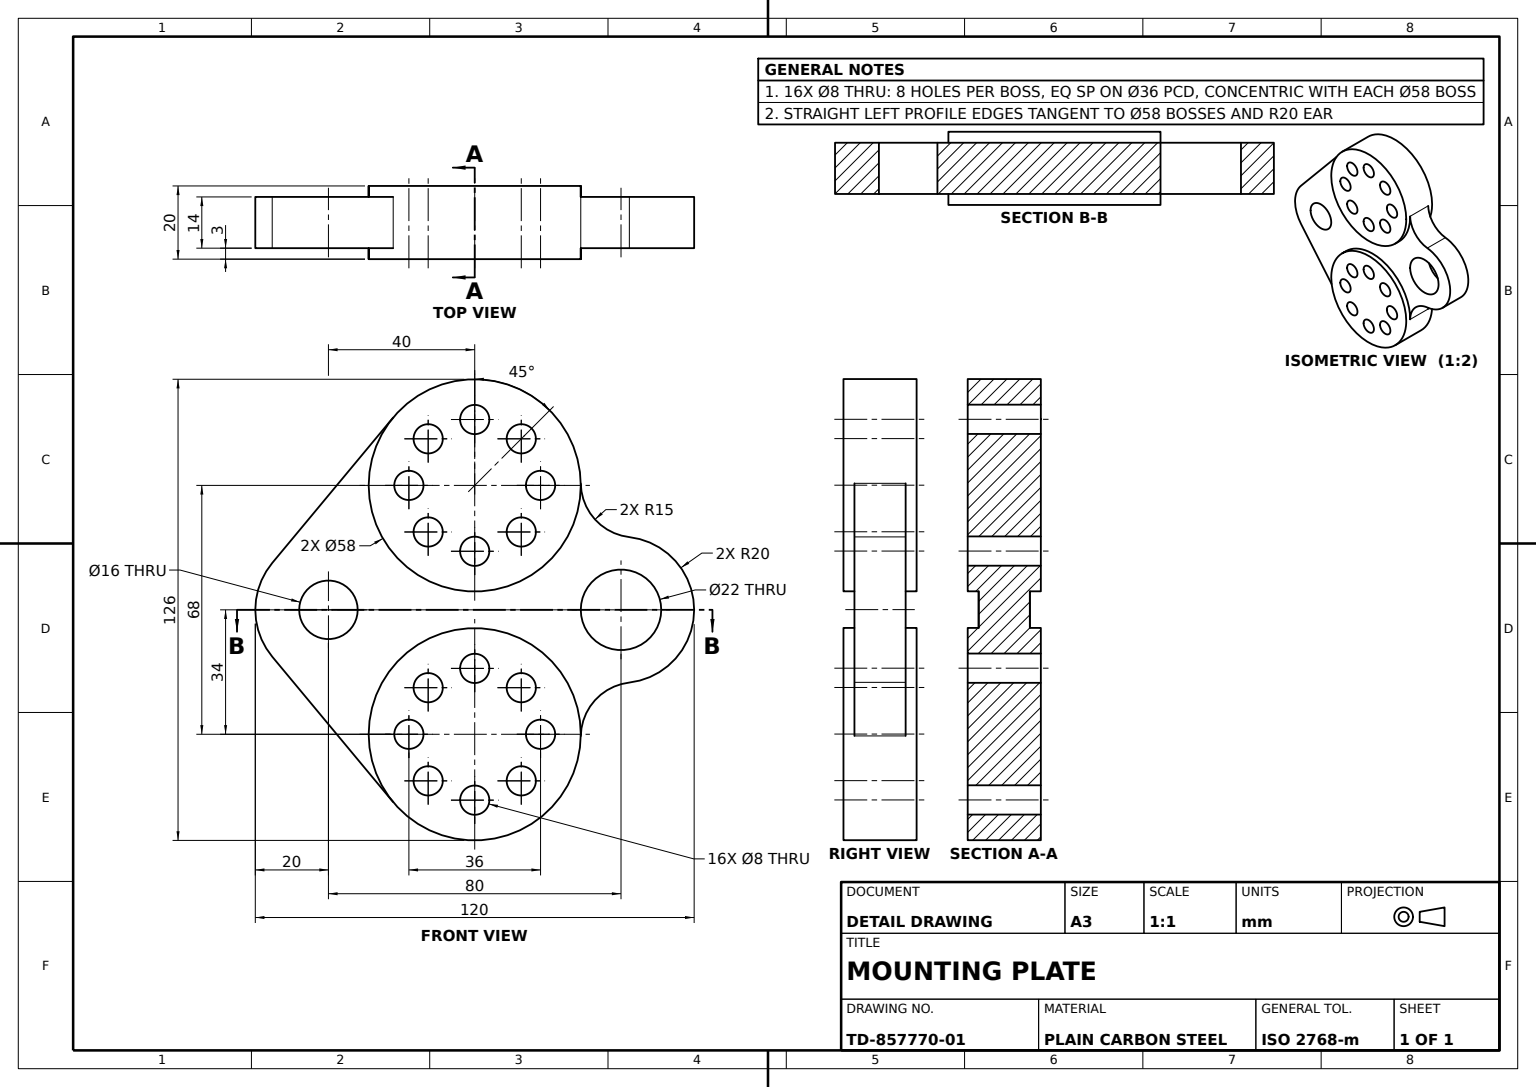
from build123d import *

# Parameters (mm, degrees)
PLATE_PROFILE_SKETCH_R      = 8
PLATE_PROFILE_SKETCH_R_2    = 11
CONNECTING_PLATE_14MM_DEPTH = 7
HUB_BOSSES_SKETCH_R         = 29
HUB_BOSSES_20MM_DEPTH       = 10
BOLT_CIRCLE_HOLES_SKETCH_R  = 4
BOLT_HOLES_2X8X_8_DEPTH     = 116.797237


with BuildPart() as part:
    # Plate Profile Sketch → Connecting Plate 14mm (new, symmetric)
    with BuildSketch(Plane.XY):
        with BuildLine():
            Line((-55.373684, -21.20743), (-22.291842, 18.549226))
            ThreePointArc((-22.291842, 18.549226), (9.623005, 27.35686), (28.995542, 0.508459))
            ThreePointArc((28.995542, 0.508459), (32.885859, -9.309525), (42.281849, -14.130597))
            ThreePointArc((42.281849, -14.130597), (60, -34), (42.281849, -53.869403))
            ThreePointArc((42.281849, -53.869403), (32.885859, -58.690475), (28.995542, -68.508459))
            ThreePointArc((28.995542, -68.508459), (9.623005, -95.35686), (-22.291842, -86.549226))
            Line((-22.291842, -86.549226), (-55.373684, -46.79257))
            ThreePointArc((-55.373684, -46.79257), (-60, -34), (-55.373684, -21.20743))
        make_face()
        with Locations((-40, -34)):
            Circle(PLATE_PROFILE_SKETCH_R, mode=Mode.SUBTRACT)
        with Locations((40, -34)):
            Circle(PLATE_PROFILE_SKETCH_R_2, mode=Mode.SUBTRACT)
    extrude(amount=CONNECTING_PLATE_14MM_DEPTH, both=True)

    # Hub Bosses Sketch → Hub Bosses 20mm (add, symmetric)
    with BuildSketch(Plane.XY):
        Circle(HUB_BOSSES_SKETCH_R)
        with Locations((0, -68)):
            Circle(HUB_BOSSES_SKETCH_R)
    extrude(amount=HUB_BOSSES_20MM_DEPTH, both=True)

    # Bolt Circle Holes Sketch → Bolt Holes 2x8xØ8 (cut, through all)
    with BuildSketch(Plane.XY.offset(10)):
        with Locations((0, 18)):
            Circle(BOLT_CIRCLE_HOLES_SKETCH_R)
        with Locations((12.727922, 12.727922)):
            Circle(BOLT_CIRCLE_HOLES_SKETCH_R)
        with Locations((18, 0)):
            Circle(BOLT_CIRCLE_HOLES_SKETCH_R)
        with Locations((12.727922, -12.727922)):
            Circle(BOLT_CIRCLE_HOLES_SKETCH_R)
        with Locations((0, -18)):
            Circle(BOLT_CIRCLE_HOLES_SKETCH_R)
        with Locations((-12.727922, -12.727922)):
            Circle(BOLT_CIRCLE_HOLES_SKETCH_R)
        with Locations((-18, 0)):
            Circle(BOLT_CIRCLE_HOLES_SKETCH_R)
        with Locations((-12.727922, 12.727922)):
            Circle(BOLT_CIRCLE_HOLES_SKETCH_R)
        with Locations((0, -50)):
            Circle(BOLT_CIRCLE_HOLES_SKETCH_R)
        with Locations((12.727922, -55.272078)):
            Circle(BOLT_CIRCLE_HOLES_SKETCH_R)
        with Locations((18, -68)):
            Circle(BOLT_CIRCLE_HOLES_SKETCH_R)
        with Locations((12.727922, -80.727922)):
            Circle(BOLT_CIRCLE_HOLES_SKETCH_R)
        with Locations((0, -86)):
            Circle(BOLT_CIRCLE_HOLES_SKETCH_R)
        with Locations((-12.727922, -80.727922)):
            Circle(BOLT_CIRCLE_HOLES_SKETCH_R)
        with Locations((-18, -68)):
            Circle(BOLT_CIRCLE_HOLES_SKETCH_R)
        with Locations((-12.727922, -55.272078)):
            Circle(BOLT_CIRCLE_HOLES_SKETCH_R)
    extrude(amount=-BOLT_HOLES_2X8X_8_DEPTH, mode=Mode.SUBTRACT)


solid = part.part
